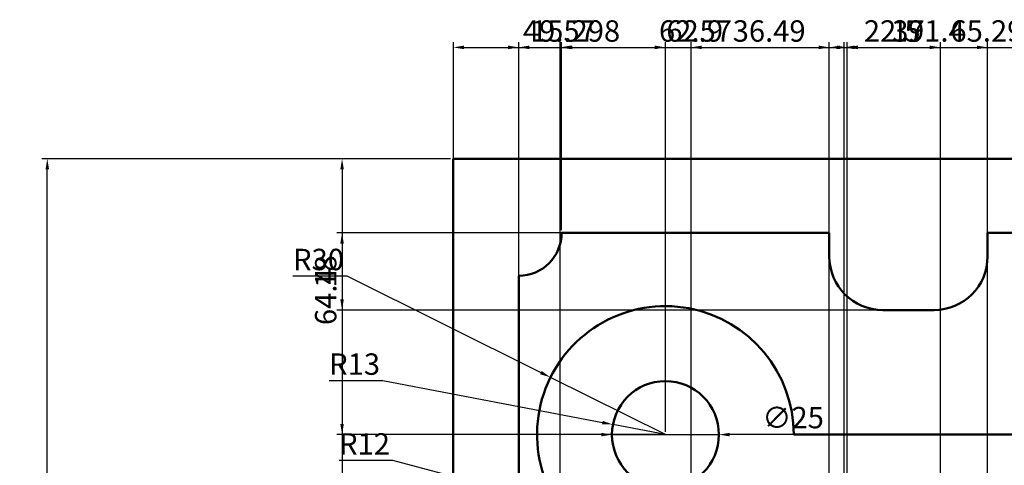
# Model space of a CAD drawing. Units: millimetres. Extents: x 1744 to 2162, y 1763 to 2334.
# Tile 4 of 5: x 1744 to 1975, y 2230 to 2334. Entities that reach past the tile are written whole.
import ezdxf

# ---------------------------------------------------------------- set-up
doc = ezdxf.new("R2010")
doc.units = ezdxf.units.MM
doc.layers.add('M-DIMS', color=2, linetype='Continuous', lineweight=25)
doc.layers.add('M-OUTL', color=7, linetype='Continuous', lineweight=50)
doc.styles.get("Standard").update_dxf_attribs({"font": 'arial.ttf'})
doc.dimstyles.new('ISO-25', dxfattribs={"dimtxt": 5, "dimasz": 2.5, "dimexe": 1.25, "dimexo": 0.625, "dimtad": 1, "dimtoh": 1, "dimdec": 0, "dimtxsty": 'Standard', "dimcen": 2.5, "dimadec": 0, "dimazin": 0, "dimtfac": 1, "dimtdec": 0, "dimtmove": 0, "dimatfit": 3, "dimfxl": 1, "dimarcsym": 0})

# ---------------------------------------------------------------- blocks, each defined once
blk = doc.blocks.new('*D1')
at = {"layer": 'Defpoints', "color": 0, "transparency": 16777216}
for p in [(1750.93, 2301.76), (1845.83, 2301.76), (1863.15, 1826.76)]:
    blk.add_point(p, dxfattribs=at)
at = {"layer": 'M-DIMS', "color": 0, "lineweight": -2, "transparency": 16777216}
for p, q in [((1845.2, 2301.76), (1749.68, 2301.76)), ((1750.93, 1829.26), (1750.93, 2299.26)), ((1862.52, 1826.76), (1749.68, 1826.76))]:
    blk.add_line(p, q, dxfattribs=at)
at = {"layer": 'M-DIMS', "color": 0, "transparency": 16777216}
for points in [[(1750.52, 2299.26), (1751.35, 2299.26), (1750.93, 2301.76)], [(1750.52, 1829.26), (1751.35, 1829.26), (1750.93, 1826.76)]]:
    blk.add_solid(points, dxfattribs=at)
at = {"layer": 'M-DIMS', "color": 0, "transparency": 16777216, "insert": (1747.76, 2064.26), "char_height": 5, "attachment_point": 5, "rotation": 90}
blk.add_mtext('475', dxfattribs=at)
blk = doc.blocks.new('*D6')
at = {"layer": 'Defpoints', "color": 0, "transparency": 16777216}
for p in [(1868.54, 2250.72), (1895.4, 2237.36)]:
    blk.add_point(p, dxfattribs=at)
at = {"layer": 'M-DIMS', "color": 0, "lineweight": -2, "transparency": 16777216}
for p, q in [((1808.35, 2274.41), (1820.91, 2274.41)), ((1820.91, 2274.41), (1866.3, 2251.83)), ((1895.4, 2237.36), (1868.54, 2250.72))]:
    blk.add_line(p, q, dxfattribs=at)
at = {"layer": 'M-DIMS', "color": 0, "transparency": 16777216}
blk.add_solid([(1866.48, 2252.21), (1866.11, 2251.46), (1868.54, 2250.72)], dxfattribs=at)
at = {"layer": 'M-DIMS', "color": 0, "transparency": 16777216, "insert": (1814.32, 2277.59), "char_height": 5, "attachment_point": 5}
blk.add_mtext('R30', dxfattribs=at)
blk = doc.blocks.new('*D7')
at = {"layer": 'Defpoints', "color": 0, "transparency": 16777216}
for p in [(1883.12, 2239.71), (1895.4, 2237.36)]:
    blk.add_point(p, dxfattribs=at)
at = {"layer": 'M-DIMS', "color": 0, "lineweight": -2, "transparency": 16777216}
for p, q in [((1816.78, 2249.99), (1829.35, 2249.99)), ((1829.35, 2249.99), (1880.66, 2240.18)), ((1895.4, 2237.36), (1883.12, 2239.71))]:
    blk.add_line(p, q, dxfattribs=at)
at = {"layer": 'M-DIMS', "color": 0, "transparency": 16777216}
blk.add_solid([(1880.74, 2240.58), (1880.59, 2239.77), (1883.12, 2239.71)], dxfattribs=at)
at = {"layer": 'M-DIMS', "color": 0, "transparency": 16777216, "insert": (1822.75, 2253.17), "char_height": 5, "attachment_point": 5}
blk.add_mtext('R13', dxfattribs=at)
blk = doc.blocks.new('*D8')
at = {"layer": 'Defpoints', "color": 0, "transparency": 16777216}
for p in [(1889.8, 2215.94), (1901.4, 2212.86)]:
    blk.add_point(p, dxfattribs=at)
at = {"layer": 'M-DIMS', "color": 0, "lineweight": -2, "transparency": 16777216}
for p, q in [((1819.12, 2231.4), (1831.64, 2231.4)), ((1831.64, 2231.4), (1887.38, 2216.58)), ((1901.4, 2212.86), (1889.8, 2215.94))]:
    blk.add_line(p, q, dxfattribs=at)
at = {"layer": 'M-DIMS', "color": 0, "transparency": 16777216}
blk.add_solid([(1887.49, 2216.99), (1887.28, 2216.18), (1889.8, 2215.94)], dxfattribs=at)
at = {"layer": 'M-DIMS', "color": 0, "transparency": 16777216, "insert": (1825.07, 2234.54), "char_height": 5, "attachment_point": 5}
blk.add_mtext('R12', dxfattribs=at)
blk = doc.blocks.new('*D29')
at = {"layer": 'Defpoints', "color": 0, "transparency": 16777216}
for p in [(2052.51, 2327.76), (2052.51, 1966.98), (1937.15, 1938.72)]:
    blk.add_point(p, dxfattribs=at)
at = {"layer": 'M-DIMS', "color": 0, "lineweight": -2, "transparency": 16777216}
for p, q in [((1937.15, 1939.34), (1937.15, 2329.01)), ((2052.51, 1967.6), (2052.51, 2329.01)), ((1939.65, 2327.76), (2050.01, 2327.76))]:
    blk.add_line(p, q, dxfattribs=at)
at = {"layer": 'M-DIMS', "color": 0, "transparency": 16777216}
for points in [[(1939.65, 2328.18), (1939.65, 2327.34), (1937.15, 2327.76)], [(2050.01, 2328.18), (2050.01, 2327.34), (2052.51, 2327.76)]]:
    blk.add_solid(points, dxfattribs=at)
at = {"layer": 'M-DIMS', "color": 0, "transparency": 16777216, "insert": (1994.83, 2330.94), "char_height": 5, "attachment_point": 5}
blk.add_mtext('115.35', dxfattribs=at)
blk = doc.blocks.new('*D30')
at = {"layer": 'Defpoints', "color": 0, "transparency": 16777216}
for p in [(1959.65, 2327.76), (1959.65, 2021.02), (1937.15, 1938.72)]:
    blk.add_point(p, dxfattribs=at)
at = {"layer": 'M-DIMS', "color": 0, "lineweight": -2, "transparency": 16777216}
for p, q in [((1937.15, 1939.34), (1937.15, 2329.01)), ((1959.65, 2021.64), (1959.65, 2329.01)), ((1939.65, 2327.76), (1957.15, 2327.76))]:
    blk.add_line(p, q, dxfattribs=at)
at = {"layer": 'M-DIMS', "color": 0, "transparency": 16777216}
for points in [[(1939.65, 2328.18), (1939.65, 2327.34), (1937.15, 2327.76)], [(1957.15, 2328.18), (1957.15, 2327.34), (1959.65, 2327.76)]]:
    blk.add_solid(points, dxfattribs=at)
at = {"layer": 'M-DIMS', "color": 0, "transparency": 16777216, "insert": (1948.4, 2330.94), "char_height": 5, "attachment_point": 5}
blk.add_mtext('22.5', dxfattribs=at)
blk = doc.blocks.new('*D33')
at = {"layer": 'Defpoints', "color": 0, "transparency": 16777216}
for p in [(1895.4, 2327.76), (1845.83, 2301.76), (1895.4, 2237.36)]:
    blk.add_point(p, dxfattribs=at)
at = {"layer": 'M-DIMS', "color": 0, "lineweight": -2, "transparency": 16777216}
for p, q in [((1845.83, 2302.39), (1845.83, 2329.01)), ((1895.4, 2237.98), (1895.4, 2329.01)), ((1848.33, 2327.76), (1892.9, 2327.76))]:
    blk.add_line(p, q, dxfattribs=at)
at = {"layer": 'M-DIMS', "color": 0, "transparency": 16777216}
for points in [[(1848.33, 2328.18), (1848.33, 2327.34), (1845.83, 2327.76)], [(1892.9, 2328.18), (1892.9, 2327.34), (1895.4, 2327.76)]]:
    blk.add_solid(points, dxfattribs=at)
at = {"layer": 'M-DIMS', "color": 0, "transparency": 16777216, "insert": (1870.61, 2330.94), "char_height": 5, "attachment_point": 5}
blk.add_mtext('49.57', dxfattribs=at)
blk = doc.blocks.new('*D34')
at = {"layer": 'Defpoints', "color": 0, "transparency": 16777216}
for p in [(2003.18, 2327.76), (2003.18, 2221.73), (1937.89, 2177.89)]:
    blk.add_point(p, dxfattribs=at)
at = {"layer": 'M-DIMS', "color": 0, "lineweight": -2, "transparency": 16777216}
for p, q in [((1937.89, 2178.51), (1937.89, 2329.01)), ((2003.18, 2222.36), (2003.18, 2329.01)), ((1940.39, 2327.76), (2000.68, 2327.76))]:
    blk.add_line(p, q, dxfattribs=at)
at = {"layer": 'M-DIMS', "color": 0, "transparency": 16777216}
for points in [[(1940.39, 2328.18), (1940.39, 2327.34), (1937.89, 2327.76)], [(2000.68, 2328.18), (2000.68, 2327.34), (2003.18, 2327.76)]]:
    blk.add_solid(points, dxfattribs=at)
at = {"layer": 'M-DIMS', "color": 0, "transparency": 16777216, "insert": (1970.53, 2330.94), "char_height": 5, "attachment_point": 5}
blk.add_mtext('65.29', dxfattribs=at)
blk = doc.blocks.new('*D36')
at = {"layer": 'Defpoints', "color": 0, "transparency": 16777216}
for p in [(1937.89, 2327.76), (1901.4, 2212.86), (1937.89, 2177.89)]:
    blk.add_point(p, dxfattribs=at)
at = {"layer": 'M-DIMS', "color": 0, "lineweight": -2, "transparency": 16777216}
for p, q in [((1901.4, 2213.48), (1901.4, 2329.01)), ((1937.89, 2178.51), (1937.89, 2329.01)), ((1903.9, 2327.76), (1935.39, 2327.76))]:
    blk.add_line(p, q, dxfattribs=at)
at = {"layer": 'M-DIMS', "color": 0, "transparency": 16777216}
for points in [[(1903.9, 2328.18), (1903.9, 2327.34), (1901.4, 2327.76)], [(1935.39, 2328.18), (1935.39, 2327.34), (1937.89, 2327.76)]]:
    blk.add_solid(points, dxfattribs=at)
at = {"layer": 'M-DIMS', "color": 0, "transparency": 16777216, "insert": (1919.64, 2330.94), "char_height": 5, "attachment_point": 5}
blk.add_mtext('36.49', dxfattribs=at)
blk = doc.blocks.new('*D38')
at = {"layer": 'Defpoints', "color": 0, "transparency": 16777216}
for p in [(1845.83, 2301.76), (1819.83, 2237.36), (1895.4, 2237.36)]:
    blk.add_point(p, dxfattribs=at)
at = {"layer": 'M-DIMS', "color": 0, "lineweight": -2, "transparency": 16777216}
for p, q in [((1845.2, 2301.76), (1818.58, 2301.76)), ((1819.83, 2299.26), (1819.83, 2239.86)), ((1894.77, 2237.36), (1818.58, 2237.36))]:
    blk.add_line(p, q, dxfattribs=at)
at = {"layer": 'M-DIMS', "color": 0, "transparency": 16777216}
for points in [[(1819.41, 2299.26), (1820.24, 2299.26), (1819.83, 2301.76)], [(1819.41, 2239.86), (1820.24, 2239.86), (1819.83, 2237.36)]]:
    blk.add_solid(points, dxfattribs=at)
at = {"layer": 'M-DIMS', "color": 0, "transparency": 16777216, "insert": (1816.65, 2269.56), "char_height": 5, "attachment_point": 5, "rotation": 90}
blk.add_mtext('64.4', dxfattribs=at)
blk = doc.blocks.new('*D46')
at = {"layer": 'Defpoints', "color": 0, "transparency": 16777216}
for p in [(2052.51, 2327.76), (1861.12, 1859.18), (2052.51, 1857.29)]:
    blk.add_point(p, dxfattribs=at)
at = {"layer": 'M-DIMS', "color": 0, "lineweight": -2, "transparency": 16777216}
for p, q in [((1861.12, 1859.81), (1861.12, 2329.01)), ((2052.51, 1857.91), (2052.51, 2329.01)), ((1863.62, 2327.76), (2050.01, 2327.76))]:
    blk.add_line(p, q, dxfattribs=at)
at = {"layer": 'M-DIMS', "color": 0, "transparency": 16777216}
for points in [[(1863.62, 2328.18), (1863.62, 2327.34), (1861.12, 2327.76)], [(2050.01, 2328.18), (2050.01, 2327.34), (2052.51, 2327.76)]]:
    blk.add_solid(points, dxfattribs=at)
at = {"layer": 'M-DIMS', "color": 0, "transparency": 16777216, "insert": (1956.82, 2330.94), "char_height": 5, "attachment_point": 5}
blk.add_mtext('191.4', dxfattribs=at)
blk = doc.blocks.new('*D47')
at = {"layer": 'Defpoints', "color": 0, "transparency": 16777216}
for p in [(1871.12, 2284.44), (1819.83, 1842.43), (1870.79, 1842.43)]:
    blk.add_point(p, dxfattribs=at)
at = {"layer": 'M-DIMS', "color": 0, "lineweight": -2, "transparency": 16777216}
for p, q in [((1870.5, 2284.44), (1818.58, 2284.44)), ((1819.83, 2281.94), (1819.83, 1844.93)), ((1870.17, 1842.43), (1818.58, 1842.43))]:
    blk.add_line(p, q, dxfattribs=at)
at = {"layer": 'M-DIMS', "color": 0, "transparency": 16777216}
for points in [[(1819.41, 2281.94), (1820.24, 2281.94), (1819.83, 2284.44)], [(1819.41, 1844.93), (1820.24, 1844.93), (1819.83, 1842.43)]]:
    blk.add_solid(points, dxfattribs=at)
at = {"layer": 'M-DIMS', "color": 0, "transparency": 16777216, "insert": (1816.69, 2063.44), "char_height": 5, "attachment_point": 5, "rotation": 90}
blk.add_mtext('442', dxfattribs=at)
blk = doc.blocks.new('*D48')
at = {"layer": 'Defpoints', "color": 0, "transparency": 16777216}
for p in [(1861.12, 2327.76), (1861.12, 1859.18), (1845.83, 1856.76)]:
    blk.add_point(p, dxfattribs=at)
at = {"layer": 'M-DIMS', "color": 0, "lineweight": -2, "transparency": 16777216}
for p, q in [((1845.83, 1857.39), (1845.83, 2329.01)), ((1861.12, 1859.81), (1861.12, 2329.01)), ((1848.33, 2327.76), (1858.62, 2327.76)), ((1861.12, 2327.76), (1885.17, 2327.76))]:
    blk.add_line(p, q, dxfattribs=at)
at = {"layer": 'M-DIMS', "color": 0, "transparency": 16777216}
for points in [[(1848.33, 2328.18), (1848.33, 2327.34), (1845.83, 2327.76)], [(1858.62, 2328.18), (1858.62, 2327.34), (1861.12, 2327.76)]]:
    blk.add_solid(points, dxfattribs=at)
at = {"layer": 'M-DIMS', "color": 0, "transparency": 16777216, "insert": (1874.4, 2330.94), "char_height": 5, "attachment_point": 5}
blk.add_mtext('15.298', dxfattribs=at)
blk = doc.blocks.new('*D50')
at = {"layer": 'Defpoints', "color": 0, "transparency": 16777216}
for p in [(1970.69, 2327.76), (1933.69, 2284.44), (1970.69, 2284.44)]:
    blk.add_point(p, dxfattribs=at)
at = {"layer": 'M-DIMS', "color": 0, "lineweight": -2, "transparency": 16777216}
for p, q in [((1933.69, 2285.06), (1933.69, 2329.01)), ((1970.69, 2285.06), (1970.69, 2329.01)), ((1936.19, 2327.76), (1968.19, 2327.76))]:
    blk.add_line(p, q, dxfattribs=at)
at = {"layer": 'M-DIMS', "color": 0, "transparency": 16777216}
for points in [[(1936.19, 2328.18), (1936.19, 2327.34), (1933.69, 2327.76)], [(1968.19, 2328.18), (1968.19, 2327.34), (1970.69, 2327.76)]]:
    blk.add_solid(points, dxfattribs=at)
at = {"layer": 'M-DIMS', "color": 0, "transparency": 16777216, "insert": (1952.19, 2330.94), "char_height": 5, "attachment_point": 5}
blk.add_mtext('37', dxfattribs=at)
blk = doc.blocks.new('*D51')
at = {"layer": 'Defpoints', "color": 0, "transparency": 16777216}
for p in [(1933.69, 2284.44), (1819.83, 2266.44), (1946.19, 2266.44)]:
    blk.add_point(p, dxfattribs=at)
at = {"layer": 'M-DIMS', "color": 0, "lineweight": -2, "transparency": 16777216}
for p, q in [((1933.07, 2284.44), (1818.58, 2284.44)), ((1819.83, 2281.94), (1819.83, 2268.94)), ((1945.57, 2266.44), (1818.58, 2266.44))]:
    blk.add_line(p, q, dxfattribs=at)
at = {"layer": 'M-DIMS', "color": 0, "transparency": 16777216}
for points in [[(1819.41, 2281.94), (1820.24, 2281.94), (1819.83, 2284.44)], [(1819.41, 2268.94), (1820.24, 2268.94), (1819.83, 2266.44)]]:
    blk.add_solid(points, dxfattribs=at)
at = {"layer": 'M-DIMS', "color": 0, "transparency": 16777216, "insert": (1816.65, 2275.44), "char_height": 5, "attachment_point": 5, "rotation": 90}
blk.add_mtext('18', dxfattribs=at)
blk = doc.blocks.new('*D52')
at = {"layer": 'Defpoints', "color": 0, "transparency": 16777216}
for p in [(1933.69, 2327.76), (1871.12, 2284.44), (1933.69, 2284.44)]:
    blk.add_point(p, dxfattribs=at)
at = {"layer": 'M-DIMS', "color": 0, "lineweight": -2, "transparency": 16777216}
for p, q in [((1871.12, 2285.06), (1871.12, 2329.01)), ((1933.69, 2285.06), (1933.69, 2329.01)), ((1873.62, 2327.76), (1931.19, 2327.76))]:
    blk.add_line(p, q, dxfattribs=at)
at = {"layer": 'M-DIMS', "color": 0, "transparency": 16777216}
for points in [[(1873.62, 2328.18), (1873.62, 2327.34), (1871.12, 2327.76)], [(1931.19, 2328.18), (1931.19, 2327.34), (1933.69, 2327.76)]]:
    blk.add_solid(points, dxfattribs=at)
at = {"layer": 'M-DIMS', "color": 0, "transparency": 16777216, "insert": (1902.41, 2330.94), "char_height": 5, "attachment_point": 5}
blk.add_mtext('62.57', dxfattribs=at)
blk = doc.blocks.new('*D60')
at = {"layer": 'Defpoints', "color": 0, "transparency": 16777216}
for p in [(1933.69, 2327.76), (1870.79, 1842.43), (1933.69, 1842.43)]:
    blk.add_point(p, dxfattribs=at)
at = {"layer": 'M-DIMS', "color": 0, "lineweight": -2, "transparency": 16777216}
for p, q in [((1870.79, 1843.06), (1870.79, 2329.01)), ((1933.69, 1843.06), (1933.69, 2329.01)), ((1873.29, 2327.76), (1931.19, 2327.76))]:
    blk.add_line(p, q, dxfattribs=at)
at = {"layer": 'M-DIMS', "color": 0, "transparency": 16777216}
for points in [[(1873.29, 2328.18), (1873.29, 2327.34), (1870.79, 2327.76)], [(1931.19, 2328.18), (1931.19, 2327.34), (1933.69, 2327.76)]]:
    blk.add_solid(points, dxfattribs=at)
at = {"layer": 'M-DIMS', "color": 0, "transparency": 16777216, "insert": (1902.24, 2330.94), "char_height": 5, "attachment_point": 5}
blk.add_mtext('62.9', dxfattribs=at)
blk = doc.blocks.new('*D61')
at = {"layer": 'Defpoints', "color": 0, "transparency": 16777216}
for p in [(1970.69, 2327.76), (1933.69, 1842.43), (1970.69, 1842.43)]:
    blk.add_point(p, dxfattribs=at)
at = {"layer": 'M-DIMS', "color": 0, "lineweight": -2, "transparency": 16777216}
for p, q in [((1933.69, 1843.06), (1933.69, 2329.01)), ((1970.69, 1843.06), (1970.69, 2329.01)), ((1936.19, 2327.76), (1968.19, 2327.76))]:
    blk.add_line(p, q, dxfattribs=at)
at = {"layer": 'M-DIMS', "color": 0, "transparency": 16777216}
for points in [[(1936.19, 2328.18), (1936.19, 2327.34), (1933.69, 2327.76)], [(1968.19, 2328.18), (1968.19, 2327.34), (1970.69, 2327.76)]]:
    blk.add_solid(points, dxfattribs=at)
at = {"layer": 'M-DIMS', "color": 0, "transparency": 16777216, "insert": (1952.19, 2330.94), "char_height": 5, "attachment_point": 5}
blk.add_mtext('37', dxfattribs=at)
blk = doc.blocks.new('*D85')
at = {"layer": 'Defpoints', "color": 0, "transparency": 16777216}
for p in [(1882.9, 2237.36), (1907.9, 2237.36)]:
    blk.add_point(p, dxfattribs=at)
at = {"layer": 'M-DIMS', "color": 0, "lineweight": -2, "transparency": 16777216}
for p, q in [((1880.4, 2237.36), (1877.9, 2237.36)), ((1882.9, 2237.36), (1907.9, 2237.36)), ((1918.28, 2237.36), (1910.4, 2237.36)), ((1931.55, 2237.36), (1918.28, 2237.36))]:
    blk.add_line(p, q, dxfattribs=at)
at = {"layer": 'M-DIMS', "color": 0, "transparency": 16777216}
for points in [[(1880.4, 2237.78), (1880.4, 2236.94), (1882.9, 2237.36)], [(1910.4, 2237.77), (1910.4, 2236.94), (1907.9, 2237.36)]]:
    blk.add_solid(points, dxfattribs=at)
at = {"layer": 'M-DIMS', "color": 0, "transparency": 16777216, "insert": (1925.23, 2240.68), "char_height": 5, "attachment_point": 5}
blk.add_mtext('∅25', dxfattribs=at)

msp = doc.modelspace()

# ---------------------------------------------------------------- linework, layer by layer
at = {"layer": 'M-OUTL'}
for p, q in [((1845.8255, 2301.7604), (1845.8255, 1856.7604)), ((1845.8255, 2301.7604), (2029.8255, 2301.7604)), ((1871.1237, 2284.4372), (1933.6942, 2284.4372)), ((1933.6942, 2284.4372), (1933.6942, 2278.9372)), ((1970.6942, 2278.9372), (1970.6942, 2284.4372)), ((1970.6942, 2284.4372), (2015.2647, 2284.4372)), ((1861.1237, 2274.4372), (1861.1237, 2172.4535)), ((1946.1942, 2266.4372), (1952.1942, 2266.4372)), ((1952.1942, 2266.4372), (1958.1942, 2266.4372)), ((2015.2647, 2237.3582), (1925.3972, 2237.3582))]:
    msp.add_line(p, q, dxfattribs=at)
msp.add_circle((1895.3972, 2237.3582), 12.5, dxfattribs=at)
for centre, radius, start, end in [((1861.1237, 2284.4372), 10, 270, 0), ((1946.1942, 2278.9372), 12.5, 180, 270), ((1958.1942, 2278.9372), 12.5, 270, 0), ((1895.3972, 2237.3582), 30, 0, 238.372386)]:
    msp.add_arc(centre, radius, start, end, dxfattribs=at)

# ---------------------------------------------------------------- dimensions: what is measured, and where the dimension line sits
at = {"layer": 'M-DIMS'}
for base, p1, p2, override, picture, middle in [((1895.3972, 2327.7604), (1845.8255, 2301.7604), (1895.3972, 2237.3582), {"dimdec": 2, "dimlfac": 1, "dimrnd": 0, "dimzin": 0, "dimdsep": 46, "dimlunit": 2}, '*D33', (1870.6113, 2330.9382)), ((1861.1237, 2327.7604), (1845.8255, 1856.7604), (1861.1237, 1859.184), {"dimdec": 3, "dimlfac": 1, "dimrnd": 0, "dimzin": 0, "dimdsep": 46, "dimlunit": 2}, '*D48', (1874.3971, 2330.9382)), ((2052.5068, 2327.7604), (1861.1237, 1859.184), (2052.5068, 1857.2889), {"dimdec": 1, "dimlfac": 1, "dimrnd": 0, "dimzin": 0, "dimdsep": 46, "dimlunit": 2}, '*D46', (1956.8153, 2330.9382)), ((1933.6942, 2327.7604), (1870.7949, 1842.4331), (1933.6942, 1842.4331), {"dimdec": 1, "dimlfac": 1, "dimrnd": 0, "dimzin": 0, "dimdsep": 46, "dimlunit": 2}, '*D60', (1902.2445, 2330.9382)), ((1933.6942, 2327.7604), (1871.1237, 2284.4372), (1933.6942, 2284.4372), {"dimdec": 2, "dimlfac": 1, "dimrnd": 0, "dimzin": 0, "dimdsep": 46, "dimlunit": 2}, '*D52', (1902.409, 2330.9382)), ((1937.8856, 2327.7604), (1901.3972, 2212.8582), (1937.8856, 2177.888), {"dimdec": 2, "dimlfac": 1, "dimrnd": 0, "dimzin": 0, "dimdsep": 46, "dimlunit": 2}, '*D36', (1919.6414, 2330.9399)), ((1970.6942, 2327.7604), (1933.6942, 2284.4372), (1970.6942, 2284.4372), {"dimdec": 0, "dimlfac": 1, "dimrnd": 0, "dimzin": 0, "dimdsep": 46, "dimlunit": 2}, '*D50', (1952.1942, 2330.9399)), ((1970.6942, 2327.7604), (1933.6942, 1842.4331), (1970.6942, 1842.4331), {"dimdec": 0, "dimlfac": 1, "dimrnd": 0, "dimzin": 0, "dimdsep": 46, "dimlunit": 2}, '*D61', (1952.1942, 2330.9399)), ((2052.5068, 2327.7604), (1937.1543, 1938.7171), (2052.5068, 1966.9753), {"dimdec": 2, "dimlfac": 1, "dimrnd": 0, "dimzin": 0, "dimdsep": 46, "dimlunit": 2}, '*D29', (1994.8306, 2330.9399)), ((1959.6543, 2327.7604), (1937.1543, 1938.7171), (1959.6543, 2021.0157), {"dimdec": 1, "dimlfac": 1, "dimrnd": 0, "dimzin": 0, "dimdsep": 46, "dimlunit": 2}, '*D30', (1948.4043, 2330.9382)), ((2003.178, 2327.7604), (1937.8856, 2177.888), (2003.178, 2221.7343), {"dimdec": 2, "dimlfac": 1, "dimrnd": 0, "dimzin": 0, "dimdsep": 46, "dimlunit": 2}, '*D34', (1970.5318, 2330.9382))]:
    dim = msp.add_linear_dim(base=base, p1=p1, p2=p2, dimstyle='ISO-25', override=override, dxfattribs=at)
    dim.commit()
    dim.dimension.update_dxf_attribs({"geometry": picture, "text_midpoint": middle})
for base, p1, p2, override, picture, middle in [((1750.9321, 2301.7604), (1863.146, 1826.7604), (1845.8255, 2301.7604), {"dimclrd": 0, "dimclre": 0, "dimclrt": 0}, '*D1', (1747.7645, 2064.2604)), ((1819.8255, 2237.3582), (1845.8255, 2301.7604), (1895.3972, 2237.3582), {"dimdec": 1, "dimlfac": 1, "dimrnd": 0, "dimzin": 0, "dimdsep": 46, "dimlunit": 2}, '*D38', (1816.6476, 2269.5593)), ((1819.8255, 2266.4372), (1933.6942, 2284.4372), (1946.1942, 2266.4372), {"dimdec": 0, "dimlfac": 1, "dimrnd": 0, "dimzin": 0, "dimdsep": 46, "dimlunit": 2}, '*D51', (1816.6476, 2275.4372)), ((1819.8255, 1842.4331), (1871.1237, 2284.4372), (1870.7949, 1842.4331), {"dimdec": 0, "dimlfac": 1, "dimrnd": 0, "dimzin": 0, "dimdsep": 46, "dimlunit": 2}, '*D47', (1816.6902, 2063.4352))]:
    dim = msp.add_linear_dim(base=base, p1=p1, p2=p2, angle=90, dimstyle='ISO-25', override=override, dxfattribs=at)
    dim.commit()
    dim.dimension.update_dxf_attribs({"geometry": picture, "text_midpoint": middle})
for center, mpoint, picture, middle in [((1895.3972, 2237.3582), (1868.5365, 2250.7187), '*D6', (1814.3157, 2274.4102)), ((1895.39722, 2237.35824), (1883.11969, 2239.70607), '*D7', (1829.34992, 2249.98846)), ((1901.3972, 2212.8582), (1889.8, 2215.9412), '*D8', (1831.6392, 2231.4026))]:
    dim = msp.add_radius_dim(center=center, mpoint=mpoint, dimstyle='ISO-25', override={"dimclrd": 0, "dimclre": 0, "dimclrt": 0}, dxfattribs=at)
    dim.commit()
    dim.dimension.update_dxf_attribs({"geometry": picture, "text_midpoint": middle, "dimtype": 164})
dim = msp.add_diameter_dim_2p(p1=(1882.8972, 2237.3585), p2=(1907.8972, 2237.358), dimstyle='ISO-25', override={"dimdec": 0, "dimlfac": 1, "dimrnd": 0, "dimzin": 0, "dimdsep": 46, "dimlunit": 2}, dxfattribs=at)
dim.commit()
dim.dimension.update_dxf_attribs({"geometry": '*D85', "text_midpoint": (1918.2826, 2237.3578), "dimtype": 163})

doc.saveas('drawing.dxf')
